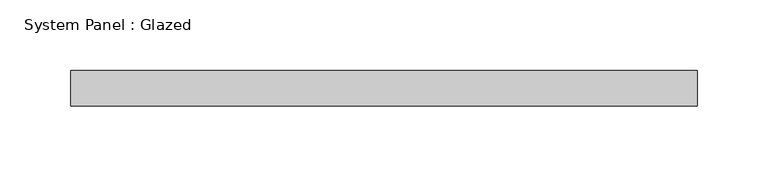
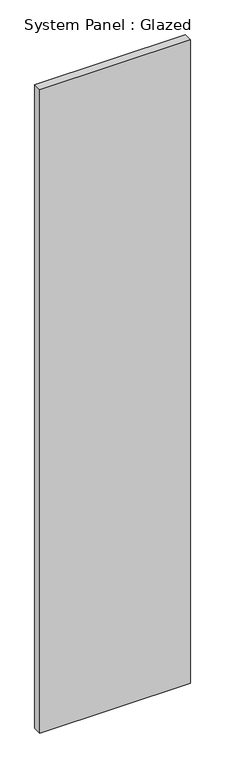
"""IFC4 building model written with IfcOpenShell, lengths in millimetres: plate geometry, System Panel : Glazed."""

from ifc_helpers import new_model, si_unit, origin, origin_with_axes, place, context, project, spatial, polyline, outline, extrude, source, transform, mapped, element, save


def system_panel_glazed_660eca69(model_context):
    return source(origin(), model_context, "Body", "SweptSolid", [
        extrude(outline(polyline([(222.25, 19.05), (-222.25, 19.05), (-222.25, 44.45), (222.25, 44.45), (222.25, 19.05)])), origin_with_axes(), (0.0, 0.0, 1.0), 2006.6),
    ])


if __name__ == "__main__":
    model = new_model("IFC4")
    model_context = context("Model", 3, world=origin())
    ifc_project = project(units=[si_unit("LENGTHUNIT", "METRE", prefix="MILLI")], contexts=[model_context])
    site = spatial("IfcSite", under=ifc_project)
    building = spatial("IfcBuilding", under=site)
    placement = place(None, origin())
    system_panel_glazed_shape = system_panel_glazed_660eca69(model_context)
    element("IfcPlate", 1, ObjectType="System Panel : Glazed", at=placement, inside=building, context=model_context, shape_type="MappedRepresentation", body=[
        mapped(system_panel_glazed_shape, transform((0.0, 0.0, 0.0), x_axis=(1.0, 0.0, 0.0), y_axis=(0.0, 1.0, 0.0), z_axis=(0.0, 0.0, 1.0))),
    ])
    save(model, "model.ifc")

# Revit data of these elements
# Type "System Panel : Glazed"
#   Construction Type Id = "GSP4R"
#   Analytic Construction = "1/8 in Pilkington single glazing"
#   Visual Light Transmittance = 0.9
#   Solar Heat Gain Coefficient = 0.86
#   Heat Transfer Coefficient (U) = 1.18115 BTU/(h·ft²·°F)
#   Define Thermal Properties by = 1
# Element 1 (IfcPlate, "System Panel : Glazed")
#   Materials on its faces: "Glass"
# Materials
#   "Glass": class "Glass", colour RGB 0 128 192, transparency 0.75, Description = "Soda Lime Glass", Cost = 0
